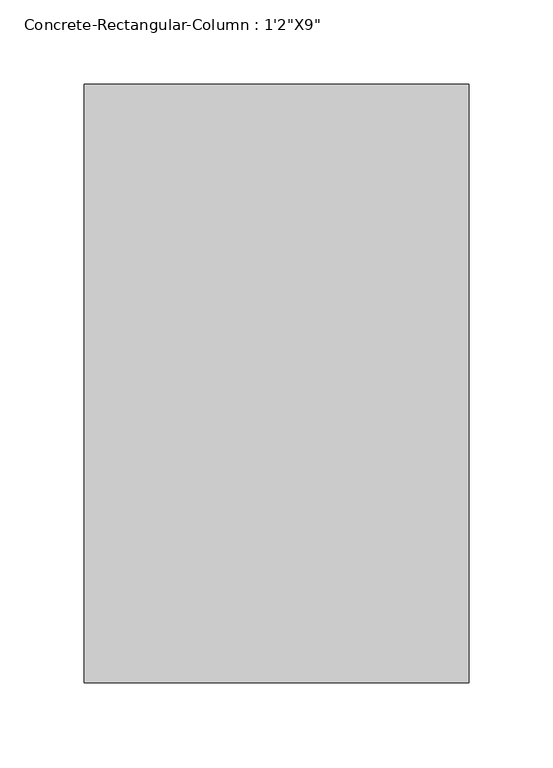
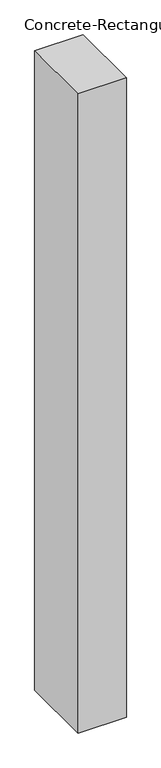
"""IFC4 building model written with IfcOpenShell, lengths in millimetres: column geometry."""

from ifc_helpers import new_model, si_unit, frame, origin, place, context, project, spatial, polyline, outline, extrude, source, transform, mapped, element, save


def column_9aa1d403(model_context):
    return source(origin(), model_context, "Body", "SweptSolid", [
        extrude(outline(polyline([(114.3, 177.8), (114.3, -177.8), (-114.3, -177.8), (-114.3, 177.8), (114.3, 177.8)])), frame((0.0, 0.0, 9601.2), z_axis=(0.0, 0.0, 1.0), x_axis=(1.0, 0.0, 0.0)), (0.0, 0.0, 1.0), 3200.4),
    ])


if __name__ == "__main__":
    model = new_model("IFC4")
    model_context = context("Model", 3, world=origin())
    ifc_project = project(units=[si_unit("LENGTHUNIT", "METRE", prefix="MILLI")], contexts=[model_context])
    site = spatial("IfcSite", under=ifc_project)
    building = spatial("IfcBuilding", under=site)
    placement = place(None, origin())
    column_shape = column_9aa1d403(model_context)
    element("IfcColumn", 1, ObjectType="Concrete-Rectangular-Column : 1'2\"X9\"", at=placement, inside=building, context=model_context, shape_type="MappedRepresentation", body=[
        mapped(column_shape, transform((0.0, 0.0, 0.0), x_axis=(1.0, 0.0, 0.0), y_axis=(0.0, 1.0, 0.0), z_axis=(0.0, 0.0, 1.0))),
    ])
    save(model, "model.ifc")

# Revit data of these elements
# Type "Concrete-Rectangular-Column : 1'2\"X9\""
#   Assembly Code = "B10"
#   b = 0' - 9"
#   h = 1' - 2"
#   Structural Material [instance default] = Concrete, Cast-in-Place gray
# Element 1 (IfcColumn, "Concrete-Rectangular-Column : 1'2\"X9\"")
#   Materials on its faces: "Concrete, Cast-in-Place gray"
# Materials
#   "Concrete, Cast-in-Place gray": class "Concrete", colour RGB 192 192 192, transparency 0, Description = "Cast-in-place concrete", Cost = 0
